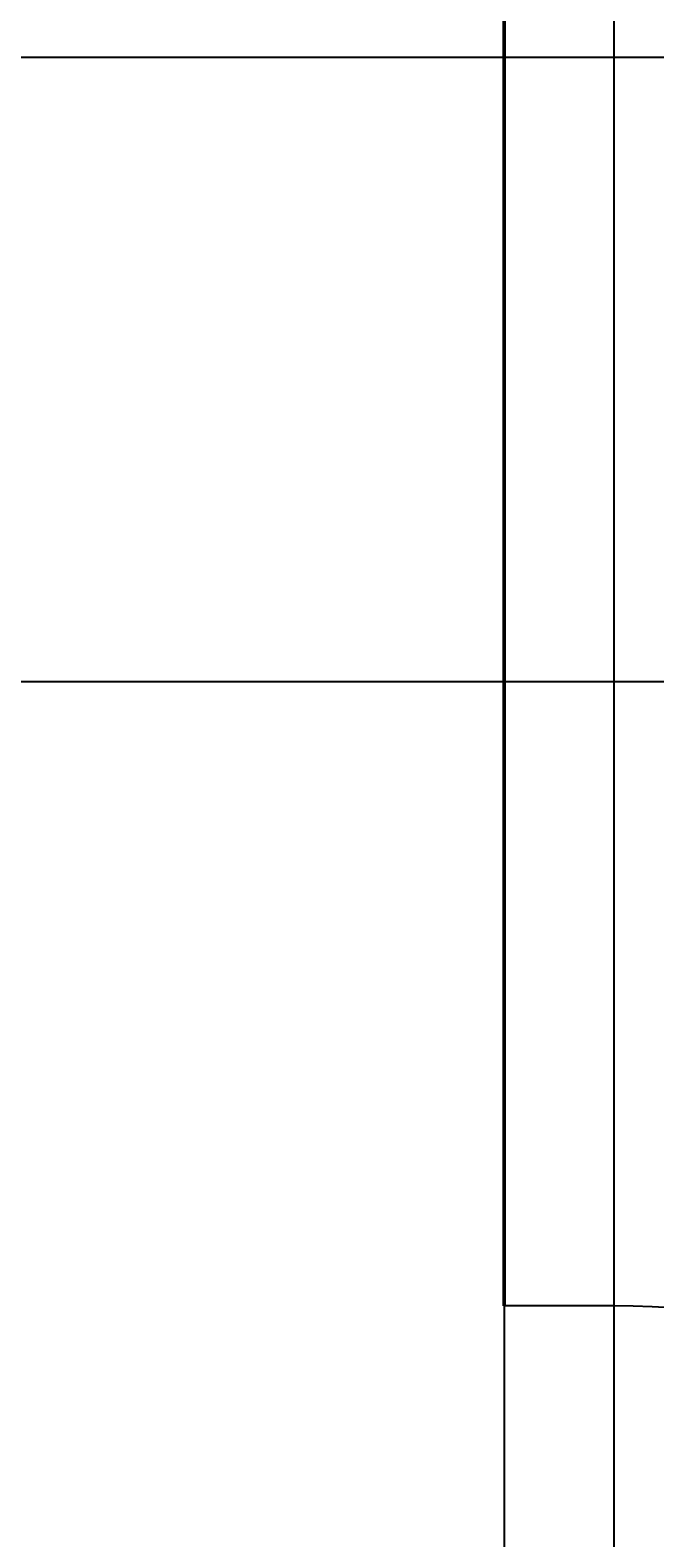
# Model space of a CAD drawing. Units: inches. Extents: x 37 to 824, y -700 to 234.
# Tile 61 of 77: x 264 to 298, y -75 to 8. Entities that reach past the tile are written whole.
import ezdxf

# ---------------------------------------------------------------- set-up
doc = ezdxf.new("R2010")
doc.units = ezdxf.units.IN
doc.header["$MEASUREMENT"] = 0
for name, color, linetype, lineweight in [('A-ANNO-DIMS', 2, 'Continuous', 18), ('A-DOOR', 4, 'Continuous', 25), ('A-WALL', 2, 'Continuous', 50)]:
    doc.layers.add(name, color=color, linetype=linetype, lineweight=lineweight)
doc.styles.get("Standard").update_dxf_attribs({"font": 'arial.ttf'})
doc.dimstyles.get("Standard").update_dxf_attribs({"dimtxt": 0.18, "dimasz": 0.18, "dimexe": 0.18, "dimexo": 0.0625, "dimgap": 0.09, "dimtad": 0, "dimtih": 1, "dimtoh": 1, "dimdec": 1, "dimzin": 0, "dimdsep": 46, "dimlunit": 4, "dimtxsty": 'Standard', "dimcen": 0.09, "dimadec": 0, "dimazin": 0, "dimtfac": 1, "dimtdec": 1, "dimtofl": 0, "dimtmove": 0, "dimatfit": 3, "dimfxl": 1, "dimtolj": 1, "dimtzin": 0, "dimarcsym": 0})

# ---------------------------------------------------------------- blocks, each defined once
blk = doc.blocks.new('*U5')
for p, q in [((0, 0), (0, 6)), ((40, 0), (40, 6))]:
    blk.add_line(p, q)
blk.add_lwpolyline([(0, 0), (0, -40), (1.75, -40), (1.75, 0)], close=True)
blk.add_arc((0, 0), 40, 270, 0)
blk = doc.blocks.new('*D62')
at = {"layer": 'A-ANNO-DIMS', "color": 0, "lineweight": -2, "ltscale": 0.5, "transparency": 16777216}
for p, q in [((419.015, 6.09), (78.159, 6.09)), ((78.339, 5.91), (78.339, -10.728)), ((78.339, -27.73), (78.339, -11.091)), ((419.015, -27.91), (78.159, -27.91))]:
    blk.add_line(p, q, dxfattribs=at)
at = {"layer": 'A-ANNO-DIMS', "color": 0, "ltscale": 0.5, "transparency": 16777216}
for points in [[(78.309, 5.91), (78.369, 5.91), (78.339, 6.09)], [(78.309, -27.73), (78.369, -27.73), (78.339, -27.91)]]:
    blk.add_solid(points, dxfattribs=at)
at = {"layer": 'Defpoints', "color": 0, "ltscale": 0.5, "transparency": 16777216}
for p in [(419.077, 6.09), (78.339, -27.91), (419.077, -27.91)]:
    blk.add_point(p, dxfattribs=at)
at = {"layer": 'A-ANNO-DIMS', "color": 0, "ltscale": 0.5, "transparency": 16777216, "insert": (78.339, -10.91), "char_height": 0.18, "attachment_point": 5}
blk.add_mtext('\\A1;2\'-10"', dxfattribs=at)
blk = doc.blocks.new('*D77')
at = {"layer": 'A-ANNO-DIMS', "color": 0, "lineweight": -2, "ltscale": 0.5, "transparency": 16777216}
for p, q in [((227.077, 45.5), (227.077, -400.406)), ((290.077, 15.028), (290.077, -400.406)), ((227.257, -400.226), (258.248, -400.226)), ((289.897, -400.226), (258.906, -400.226))]:
    blk.add_line(p, q, dxfattribs=at)
at = {"layer": 'A-ANNO-DIMS', "color": 0, "ltscale": 0.5, "transparency": 16777216}
for points in [[(227.257, -400.196), (227.257, -400.256), (227.077, -400.226)], [(289.897, -400.196), (289.897, -400.256), (290.077, -400.226)]]:
    blk.add_solid(points, dxfattribs=at)
at = {"layer": 'Defpoints', "color": 0, "ltscale": 0.5, "transparency": 16777216}
for p in [(227.077, 45.563), (290.077, 15.09), (290.077, -400.226)]:
    blk.add_point(p, dxfattribs=at)
at = {"layer": 'A-ANNO-DIMS', "color": 0, "ltscale": 0.5, "transparency": 16777216, "insert": (258.577, -400.226), "char_height": 0.18, "attachment_point": 5}
blk.add_mtext('\\A1;5\'-3"', dxfattribs=at)
blk = doc.blocks.new('*D79')
at = {"layer": 'A-ANNO-DIMS', "color": 0, "lineweight": -2, "ltscale": 0.5, "transparency": 16777216}
for p, q in [((299.14, -62.022), (513.773, -62.022)), ((513.593, -62.202), (513.593, -81.784)), ((513.593, -101.73), (513.593, -82.148)), ((296.14, -101.91), (513.773, -101.91))]:
    blk.add_line(p, q, dxfattribs=at)
at = {"layer": 'A-ANNO-DIMS', "color": 0, "ltscale": 0.5, "transparency": 16777216}
for points in [[(513.563, -62.202), (513.623, -62.202), (513.593, -62.022)], [(513.563, -101.73), (513.623, -101.73), (513.593, -101.91)]]:
    blk.add_solid(points, dxfattribs=at)
at = {"layer": 'Defpoints', "color": 0, "ltscale": 0.5, "transparency": 16777216}
for p in [(299.077, -62.022), (296.077, -101.91), (513.593, -101.91)]:
    blk.add_point(p, dxfattribs=at)
at = {"layer": 'A-ANNO-DIMS', "color": 0, "ltscale": 0.5, "transparency": 16777216, "insert": (513.593, -81.966), "char_height": 0.18, "attachment_point": 5}
blk.add_mtext('\\A1;3\'-4"', dxfattribs=at)
blk = doc.blocks.new('*D87')
at = {"layer": 'A-ANNO-DIMS', "color": 0, "lineweight": -2, "ltscale": 0.5, "transparency": 16777216}
for p, q in [((216.077, -356.847), (216.077, 234.17)), ((296.077, -356.847), (296.077, 234.17)), ((216.257, 233.99), (255.747, 233.99)), ((295.897, 233.99), (256.407, 233.99))]:
    blk.add_line(p, q, dxfattribs=at)
at = {"layer": 'A-ANNO-DIMS', "color": 0, "ltscale": 0.5, "transparency": 16777216}
for points in [[(216.257, 234.02), (216.257, 233.96), (216.077, 233.99)], [(295.897, 234.02), (295.897, 233.96), (296.077, 233.99)]]:
    blk.add_solid(points, dxfattribs=at)
at = {"layer": 'Defpoints', "color": 0, "ltscale": 0.5, "transparency": 16777216}
for p in [(296.077, 233.99), (216.077, -356.91), (296.077, -356.91)]:
    blk.add_point(p, dxfattribs=at)
at = {"layer": 'A-ANNO-DIMS', "color": 0, "ltscale": 0.5, "transparency": 16777216, "insert": (256.077, 233.99), "char_height": 0.18, "attachment_point": 5}
blk.add_mtext('\\A1;6\'-8"', dxfattribs=at)

msp = doc.modelspace()

# ---------------------------------------------------------------- linework, layer by layer
at = {"layer": 'A-WALL'}
msp.add_line((290.077, -61.91), (290.077, 15.09), dxfattribs=at)

# ---------------------------------------------------------------- block references
at = {"layer": 'A-DOOR', "rotation": 90}
msp.add_blockref('*U5', (296.077, -101.91), dxfattribs=at)

# ---------------------------------------------------------------- dimensions: what is measured, and where the dimension line sits
at = {"layer": 'A-ANNO-DIMS', "ltscale": 0.5}
for base, p1, p2, picture, middle in [((296.077, 233.99), (216.077, -356.91), (296.077, -356.91), '*D87', (256.077, 233.99)), ((290.077, -400.226), (227.077, 45.563), (290.077, 15.09), '*D77', (258.577, -400.226))]:
    dim = msp.add_linear_dim(base=base, p1=p1, p2=p2, dimstyle='Standard', override={"dimdec": 1, "dimlfac": 1, "dimrnd": 0, "dimzin": 1, "dimdsep": 46, "dimlunit": 4, "dimfrac": 2}, dxfattribs=at)
    dim.commit()
    dim.dimension.update_dxf_attribs({"geometry": picture, "text_midpoint": middle})
for base, p1, p2, picture, middle in [((78.339, -27.91), (419.077, 6.09), (419.077, -27.91), '*D62', (78.339, -10.91)), ((513.593, -101.91), (299.077, -62.022), (296.077, -101.91), '*D79', (513.593, -81.966))]:
    dim = msp.add_linear_dim(base=base, p1=p1, p2=p2, angle=90, dimstyle='Standard', override={"dimdec": 1, "dimlfac": 1, "dimrnd": 0, "dimzin": 1, "dimdsep": 46, "dimlunit": 4, "dimfrac": 2}, dxfattribs=at)
    dim.commit()
    dim.dimension.update_dxf_attribs({"geometry": picture, "text_midpoint": middle})

doc.saveas('drawing.dxf')
